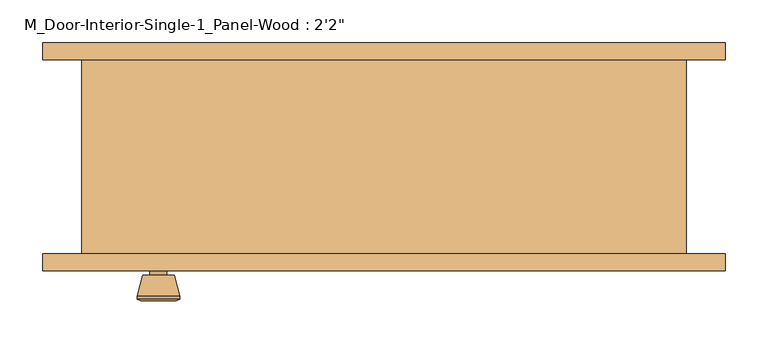
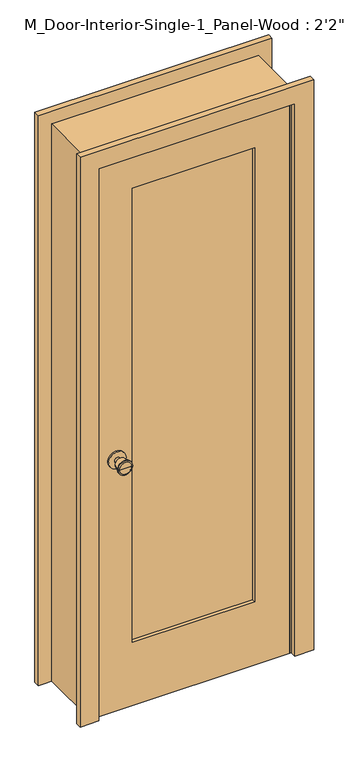
"""IFC4 building model written with IfcOpenShell, lengths in millimetres: door geometry."""

from ifc_helpers import new_model, si_unit, point, frame, frame_2d, origin, place, context, project, spatial, polyline, circle_curve, trimmed, segment, composite_curve, outline, extrude, faceted_brep, source, transform, mapped, element, save
from ifc_brep_helpers import plane_surface, cylinder_surface, revolved_surface, advanced_brep


def door_a93bef0d(model_context):
    return source(origin(), model_context, "Body", "SolidModel", [
        advanced_brep(
        [(-265.2, -70.125, 914.4), (-275.2, -70.125, 914.4), (-255.2, -70.125, 914.4), (-244.7241324, -21.125, 914.4), (-285.6758676, -21.125, 914.4), (-265.2, -21.125, 914.4), (-240.2, -22.9528681, 914.4), (-290.2, -22.9528681, 914.4), (-240.2, -26.4165463, 914.4), (-290.2, -26.4165463, 914.4), (-246.563764, -51.125, 914.4), (-283.836236, -51.125, 914.4), (-255.2, -51.125, 914.4), (-275.2, -51.125, 914.4)],
        [
            (0, 1),
            (1, 2, circle_curve(frame((-265.2, -70.125, 914.4), z_axis=(0.0, -1.0, 0.0), x_axis=(-1.0, 0.0, 0.0)), 10.0)),
            (2, 0),
            (2, 1, circle_curve(frame((-265.2, -70.125, 914.4), z_axis=(0.0, -1.0, 0.0), x_axis=(-1.0, 0.0, 0.0)), 10.0)),
            (3, 4, circle_curve(frame((-265.2, -21.125, 914.4), z_axis=(0.0, 1.0, 0.0), x_axis=(-1.0, 0.0, 0.0)), 20.4758676)),
            (4, 5),
            (5, 3),
            (4, 3, circle_curve(frame((-265.2, -21.125, 914.4), z_axis=(0.0, 1.0, 0.0), x_axis=(-1.0, 0.0, 0.0)), 20.4758676)),
            (6, 7, circle_curve(frame((-265.2, -22.9528681, 914.4), z_axis=(0.0, 1.0, 0.0), x_axis=(-1.0, 0.0, 0.0)), 25.0)),
            (7, 4),
            (3, 6),
            (7, 6, circle_curve(frame((-265.2, -22.9528681, 914.4), z_axis=(0.0, 1.0, 0.0), x_axis=(-1.0, 0.0, 0.0)), 25.0)),
            (8, 9, circle_curve(frame((-265.2, -26.4165463, 914.4), z_axis=(0.0, 1.0, 0.0), x_axis=(-1.0, 0.0, 0.0)), 25.0)),
            (9, 7),
            (6, 8),
            (9, 8, circle_curve(frame((-265.2, -26.4165463, 914.4), z_axis=(0.0, 1.0, 0.0), x_axis=(-1.0, 0.0, 0.0)), 25.0)),
            (10, 11, circle_curve(frame((-265.2, -51.125, 914.4), z_axis=(0.0, 1.0, 0.0), x_axis=(-1.0, 0.0, 0.0)), 18.636236)),
            (11, 9),
            (8, 10),
            (11, 10, circle_curve(frame((-265.2, -51.125, 914.4), z_axis=(0.0, 1.0, 0.0), x_axis=(-1.0, 0.0, 0.0)), 18.636236)),
            (12, 13, circle_curve(frame((-265.2, -51.125, 914.4), z_axis=(0.0, 1.0, 0.0), x_axis=(-1.0, 0.0, 0.0)), 10.0)),
            (13, 11),
            (10, 12),
            (13, 12, circle_curve(frame((-265.2, -51.125, 914.4), z_axis=(0.0, 1.0, 0.0), x_axis=(-1.0, 0.0, 0.0)), 10.0)),
            (1, 13),
            (12, 2),
        ],
        [
            plane_surface(frame((-265.2, -70.125, 914.4), z_axis=(0.0, -1.0, 0.0), x_axis=(-1.0, 0.0, 0.0))),
            plane_surface(frame((-265.2, -21.125, 914.4), z_axis=(0.0, 1.0, 0.0), x_axis=(-1.0, 0.0, 0.0))),
            revolved_surface(polyline([(-285.6758676, -21.125, 914.4), (-290.2, -22.9528681, 914.4)]), (-265.2, -70.125, 914.4), (0.0, -1.0, 0.0)),
            cylinder_surface(frame((-265.2, -70.125, 914.4), z_axis=(0.0, -1.0, 0.0), x_axis=(-1.0, 0.0, 0.0)), 25.0),
            revolved_surface(polyline([(-290.2, -26.4165463, 914.4), (-283.836236, -51.125, 914.4)]), (-265.2, -70.125, 914.4), (0.0, -1.0, 0.0)),
            plane_surface(frame((-265.2, -51.125, 914.4), z_axis=(0.0, -1.0, 0.0), x_axis=(-1.0, 0.0, 0.0))),
            cylinder_surface(frame((-265.2, -70.125, 914.4), z_axis=(0.0, -1.0, 0.0), x_axis=(-1.0, 0.0, 0.0)), 10.0),
        ],
        [
            (0, [[1, 2, 3]]),
            (0, [[-3, 4, -1]]),
            (1, [[5, 6, 7]]),
            (1, [[8, -7, -6]]),
            (2, [[9, 10, -5, 11]]),
            (2, [[12, -11, -8, -10]]),
            (3, [[13, 14, -9, 15]]),
            (3, [[16, -15, -12, -14]]),
            (4, [[17, 18, -13, 19]]),
            (4, [[20, -19, -16, -18]]),
            (5, [[21, 22, -17, 23]]),
            (5, [[24, -23, -20, -22]]),
            (6, [[-2, 25, -21, 26]]),
            (6, [[-4, -26, -24, -25]]),
        ],
    ),
        extrude(outline(composite_curve([segment(trimmed(circle_curve(frame_2d((914.4, -265.2)), 30.0), [point((914.4, -295.2))], [point((914.4, -235.2))], False, "CARTESIAN"), True, "CONTINUOUS"), segment(trimmed(circle_curve(frame_2d((914.4, -265.2)), 30.0), [point((914.4, -235.2))], [point((914.4, -295.2))], False, "CARTESIAN"), True, "CONTINUOUS")], self_intersect=False)), frame((0.0, -76.125, 0.0), z_axis=(0.0, 1.0, 0.0), x_axis=(0.0, 0.0, 1.0)), (0.0, 0.0, 1.0), 6.0),
        advanced_brep(
        [(-265.2, -117.125, 914.4), (-255.2, -117.125, 914.4), (-275.2, -117.125, 914.4), (-244.7241324, -166.125, 914.4), (-265.2, -166.125, 914.4), (-285.6758676, -166.125, 914.4), (-240.2, -164.2971319, 914.4), (-290.2, -164.2971319, 914.4), (-240.2, -160.8334537, 914.4), (-290.2, -160.8334537, 914.4), (-246.563764, -136.125, 914.4), (-283.836236, -136.125, 914.4), (-255.2, -136.125, 914.4), (-275.2, -136.125, 914.4)],
        [
            (0, 1),
            (1, 2, circle_curve(frame((-265.2, -117.125, 914.4), z_axis=(0.0, 1.0, 0.0), x_axis=(-1.0, 0.0, 0.0)), 10.0)),
            (2, 0),
            (2, 1, circle_curve(frame((-265.2, -117.125, 914.4), z_axis=(0.0, 1.0, 0.0), x_axis=(-1.0, 0.0, 0.0)), 10.0)),
            (3, 4),
            (4, 5),
            (5, 3, circle_curve(frame((-265.2, -166.125, 914.4), z_axis=(0.0, -1.0, 0.0), x_axis=(-1.0, 0.0, 0.0)), 20.4758676)),
            (3, 5, circle_curve(frame((-265.2, -166.125, 914.4), z_axis=(0.0, -1.0, 0.0), x_axis=(-1.0, 0.0, 0.0)), 20.4758676)),
            (6, 3),
            (5, 7),
            (7, 6, circle_curve(frame((-265.2, -164.2971319, 914.4), z_axis=(0.0, -1.0, 0.0), x_axis=(-1.0, 0.0, 0.0)), 25.0)),
            (6, 7, circle_curve(frame((-265.2, -164.2971319, 914.4), z_axis=(0.0, -1.0, 0.0), x_axis=(-1.0, 0.0, 0.0)), 25.0)),
            (8, 6),
            (7, 9),
            (9, 8, circle_curve(frame((-265.2, -160.8334537, 914.4), z_axis=(0.0, -1.0, 0.0), x_axis=(-1.0, 0.0, 0.0)), 25.0)),
            (8, 9, circle_curve(frame((-265.2, -160.8334537, 914.4), z_axis=(0.0, -1.0, 0.0), x_axis=(-1.0, 0.0, 0.0)), 25.0)),
            (10, 8),
            (9, 11),
            (11, 10, circle_curve(frame((-265.2, -136.125, 914.4), z_axis=(0.0, -1.0, 0.0), x_axis=(-1.0, 0.0, 0.0)), 18.636236)),
            (10, 11, circle_curve(frame((-265.2, -136.125, 914.4), z_axis=(0.0, -1.0, 0.0), x_axis=(-1.0, 0.0, 0.0)), 18.636236)),
            (12, 10),
            (11, 13),
            (13, 12, circle_curve(frame((-265.2, -136.125, 914.4), z_axis=(0.0, -1.0, 0.0), x_axis=(-1.0, 0.0, 0.0)), 10.0)),
            (12, 13, circle_curve(frame((-265.2, -136.125, 914.4), z_axis=(0.0, -1.0, 0.0), x_axis=(-1.0, 0.0, 0.0)), 10.0)),
            (1, 12),
            (13, 2),
        ],
        [
            plane_surface(frame((-265.2, -117.125, 914.4), z_axis=(0.0, 1.0, 0.0), x_axis=(-1.0, 0.0, 0.0))),
            plane_surface(frame((-265.2, -166.125, 914.4), z_axis=(0.0, -1.0, 0.0), x_axis=(-1.0, 0.0, 0.0))),
            revolved_surface(polyline([(-285.6758676, -166.125, 914.4), (-290.2, -164.2971319, 914.4)]), (-265.2, -117.125, 914.4), (0.0, 1.0, 0.0)),
            cylinder_surface(frame((-265.2, -117.125, 914.4), z_axis=(0.0, 1.0, 0.0), x_axis=(-1.0, 0.0, 0.0)), 25.0),
            revolved_surface(polyline([(-290.2, -160.8334537, 914.4), (-283.836236, -136.125, 914.4)]), (-265.2, -117.125, 914.4), (0.0, 1.0, 0.0)),
            plane_surface(frame((-265.2, -136.125, 914.4), z_axis=(0.0, 1.0, 0.0), x_axis=(-1.0, 0.0, 0.0))),
            cylinder_surface(frame((-265.2, -117.125, 914.4), z_axis=(0.0, 1.0, 0.0), x_axis=(-1.0, 0.0, 0.0)), 10.0),
        ],
        [
            (0, [[1, 2, 3]]),
            (0, [[-3, 4, -1]]),
            (1, [[5, 6, 7]]),
            (1, [[-6, -5, 8]]),
            (2, [[9, -7, 10, 11]]),
            (2, [[-10, -8, -9, 12]]),
            (3, [[13, -11, 14, 15]]),
            (3, [[-14, -12, -13, 16]]),
            (4, [[17, -15, 18, 19]]),
            (4, [[-18, -16, -17, 20]]),
            (5, [[21, -19, 22, 23]]),
            (5, [[-22, -20, -21, 24]]),
            (6, [[25, -23, 26, -2]]),
            (6, [[-26, -24, -25, -4]]),
        ],
    ),
        extrude(outline(composite_curve([segment(trimmed(circle_curve(frame_2d((914.4, -265.2)), 30.0), [point((914.4, -295.2))], [point((914.4, -235.2))], False, "CARTESIAN"), True, "CONTINUOUS"), segment(trimmed(circle_curve(frame_2d((914.4, -265.2)), 30.0), [point((914.4, -235.2))], [point((914.4, -295.2))], False, "CARTESIAN"), True, "CONTINUOUS")], self_intersect=False)), frame((0.0, -117.125, 0.0), z_axis=(0.0, 1.0, 0.0), x_axis=(0.0, 0.0, 1.0)), (0.0, 0.0, 1.0), 6.0),
        faceted_brep([(355.2, -111.125, 0.0), (330.2, -111.125, 0.0), (330.2, -76.125, 0.0), (317.5, -76.125, 0.0), (317.5, -41.2, 0.0), (330.2, -41.2, 0.0), (330.2, 117.475, 0.0), (355.2, 117.475, 0.0), (355.2, 117.475, 2025.0), (355.2, -111.125, 2025.0), (330.2, 117.475, 2000.0), (-330.2, 117.475, 2000.0), (-330.2, 117.475, 0.0), (-355.2, 117.475, 0.0), (-355.2, 117.475, 2025.0), (330.2, -41.2, 2000.0), (317.5, -41.2, 1987.3), (-317.5, -41.2, 1987.3), (-317.5, -41.2, 0.0), (-330.2, -41.2, 0.0), (-330.2, -41.2, 2000.0), (317.5, -76.125, 1987.3), (330.2, -76.125, 2000.0), (-330.2, -76.125, 2000.0), (-330.2, -76.125, 0.0), (-317.5, -76.125, 0.0), (-317.5, -76.125, 1987.3), (330.2, -111.125, 2000.0), (-355.2, -111.125, 2025.0), (-355.2, -111.125, 0.0), (-330.2, -111.125, 0.0), (-330.2, -111.125, 2000.0)], [[[0, 1, 2, 3, 4, 5, 6, 7]], [[7, 8, 9, 0]], [[6, 10, 11, 12, 13, 14, 8, 7]], [[5, 15, 10, 6]], [[4, 16, 17, 18, 19, 20, 15, 5]], [[3, 21, 16, 4]], [[2, 22, 23, 24, 25, 26, 21, 3]], [[1, 27, 22, 2]], [[0, 9, 28, 29, 30, 31, 27, 1]], [[8, 14, 28, 9]], [[15, 20, 11, 10]], [[21, 26, 17, 16]], [[27, 31, 23, 22]], [[29, 13, 12, 19, 18, 25, 24, 30]], [[14, 13, 29, 28]], [[20, 19, 12, 11]], [[26, 25, 18, 17]], [[31, 30, 24, 23]]]),
        extrude(outline(polyline([(2000.0, -330.2), (0.0, -330.2), (0.0, 330.2), (2000.0, 330.2), (2000.0, -330.2)]), holes=[polyline([(1880.0, -210.2), (1880.0, 210.2), (230.0, 210.2), (230.0, -210.2), (1880.0, -210.2)])]), frame((0.0, -111.125, 0.0), z_axis=(0.0, 1.0, 0.0), x_axis=(0.0, 0.0, 1.0)), (0.0, 0.0, 1.0), 35.0),
        extrude(outline(polyline([(210.2, -87.7916667), (210.2, -99.4583333), (-210.2, -99.4583333), (-210.2, -87.7916667), (210.2, -87.7916667)])), frame((0.0, 0.0, 230.0), z_axis=(0.0, 0.0, 1.0), x_axis=(1.0, 0.0, 0.0)), (0.0, 0.0, 1.0), 1650.0),
        extrude(outline(polyline([(0.0, 401.55), (2071.35, 401.55), (2071.35, -401.55), (0.0, -401.55), (0.0, -336.55), (2006.35, -336.55), (2006.35, 336.55), (0.0, 336.55), (0.0, 401.55)])), frame((0.0, -131.125, 0.0), z_axis=(0.0, 1.0, 0.0), x_axis=(0.0, 0.0, 1.0)), (0.0, 0.0, 1.0), 20.0),
        extrude(outline(polyline([(0.0, 401.55), (2071.35, 401.55), (2071.35, -401.55), (0.0, -401.55), (0.0, -336.55), (2006.35, -336.55), (2006.35, 336.55), (0.0, 336.55), (0.0, 401.55)])), frame((0.0, 117.475, 0.0), z_axis=(0.0, 1.0, 0.0), x_axis=(0.0, 0.0, 1.0)), (0.0, 0.0, 1.0), 20.0),
    ])


if __name__ == "__main__":
    model = new_model("IFC4")
    model_context = context("Model", 3, world=origin())
    ifc_project = project(units=[si_unit("LENGTHUNIT", "METRE", prefix="MILLI")], contexts=[model_context])
    site = spatial("IfcSite", under=ifc_project)
    building = spatial("IfcBuilding", under=site)
    placement = place(None, origin())
    door_shape = door_a93bef0d(model_context)
    element("IfcDoor", 1, ObjectType="M_Door-Interior-Single-1_Panel-Wood : 2'2\"", at=placement, inside=building, context=model_context, shape_type="MappedRepresentation", body=[
        mapped(door_shape, transform((0.0, 0.0, 0.0), x_axis=(1.0, 0.0, 0.0), y_axis=(0.0, 1.0, 0.0), z_axis=(0.0, 0.0, 1.0))),
    ])
    save(model, "model.ifc")

# Revit data of these elements
# Type "M_Door-Interior-Single-1_Panel-Wood : 2'2\""
#   Type Mark = "17"
#   Assembly Code = "C1020300"
#   Analytic Construction = "Wooden"
#   Top Rail = 0' - 4.72441"
#   Thickness = 0' - 1.37795"
#   Thermal Resistance (R) = 2.5876 (h·ft²·°F)/BTU
#   Swing Angle [instance default] = 90.00°
#   Stiles = 0' - 4.72441"
#   Rough Width = 2' - 3.9685"
#   Rough Height = 6' - 7.72441"
#   Height = 6' - 6.74016"
#   Width = 2' - 2"
#   Heat Transfer Coefficient (U) = 0.3865 BTU/(h·ft²·°F)
#   Bottom Rail = 0' - 9.05512"
#   Trim Material = Cherry
#   Panel Material = Cherry
#   Frame Material = Cherry
#   Door Handle Material = Aluminum
#   Visual Light Transmittance = 0
#   Solar Heat Gain Coefficient = 0
#   Wall Closure = (empty or 0)
#   Function = (empty or 0)
# Element 1 (IfcDoor, "M_Door-Interior-Single-1_Panel-Wood : 2'2\"")
#   Materials on its faces: "Cherry", "Aluminum"
# Materials
#   "Cherry": class "Wood", colour RGB 226 177 128, transparency 0, Description = "Prunus Serotina", Cost = 0
#   "Aluminum": class "Metal", colour RGB 247 247 247, transparency 0, Description = "Aluminum 6061", Cost = 0
